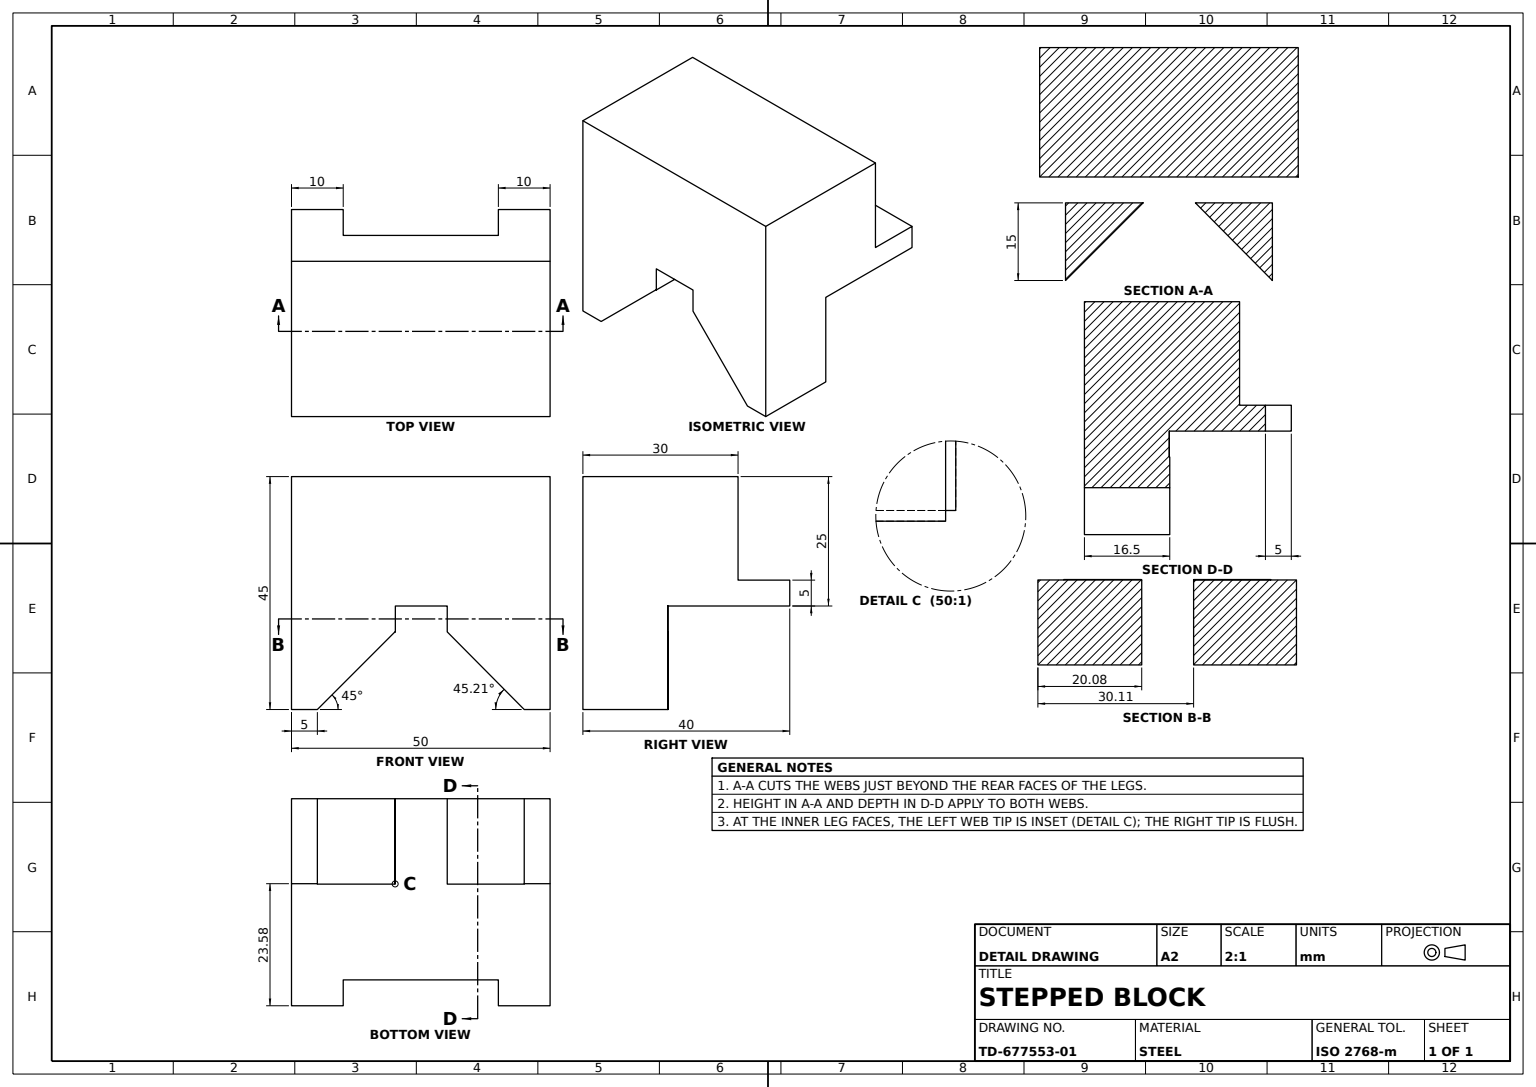
from build123d import *

# Parameters (mm, degrees)
BASE_BLOCK_SKETCH_W       = 50
BASE_BLOCK_SKETCH_H       = 30
BASE_BLOCK_50X30X25_DEPTH = 25
CORNER_STEP_5MM_DEPTH     = 5
LOWER_PLATE_SKETCH_W      = 19.888158271
LOWER_PLATE_SKETCH_H      = 16.417205811
LOWER_PLATE_5MM_DEPTH     = 5
LEG_SKETCH_W              = 5
LEG_SKETCH_H              = 16.417205811
LEG_15MM_DEPTH            = 15
TAPERED_WEB_16_5MM_DEPTH  = 16.5


with BuildPart() as part:
    # Base Block Sketch → Base Block 50x30x25 (new body)
    with BuildSketch(Plane(origin=(0, 0, 0), x_dir=(1, 0, 0), z_dir=(0, 1, 0))):
        with Locations((25, 15)):
            Rectangle(BASE_BLOCK_SKETCH_W, BASE_BLOCK_SKETCH_H)
    extrude(amount=BASE_BLOCK_50X30X25_DEPTH)

    # Corner Step Sketch → Corner Step 5mm (add)
    with BuildSketch(Plane(origin=(0, 0, 0), x_dir=(1, 0, 0), z_dir=(0, 1, 0))):
        Polygon((0, 30), (0, 40), (10, 40), (10, 35), (40, 35), (40, 40), (50, 40), (50, 30), (50, 0), (0, 0), align=None)
    extrude(amount=CORNER_STEP_5MM_DEPTH)

    # Lower Plate Sketch → Lower Plate 5mm (add)
    with BuildSketch(Plane.XZ):
        Polygon((6.770734002, 0), (0, 0), (0, -16.417205811), (6.770734002, -16.417205811), (20.078313967, -16.417205811), (20.078313967, 0), align=None)
        with Locations((40.055920865, -8.208602906)):
            Rectangle(LOWER_PLATE_SKETCH_W, LOWER_PLATE_SKETCH_H)
    extrude(amount=LOWER_PLATE_5MM_DEPTH)

    # Leg Sketch → Leg 15mm (add)
    with BuildSketch(Plane(origin=(0, -5, 0), x_dir=(-1, 0, 0), z_dir=(0, -1, 0))):
        with Locations((-2.5, 8.208602906)):
            Rectangle(LEG_SKETCH_W, LEG_SKETCH_H)
        with Locations((-47.5, 8.208602906)):
            Rectangle(LEG_SKETCH_W, LEG_SKETCH_H)
    extrude(amount=LEG_15MM_DEPTH)

    # Tapered Web Sketch → Tapered Web 16.5mm (add)
    with BuildSketch(Plane.XY):
        Polygon((30.111841729, -5), (45, -20), (45, -5), align=None)
        Polygon((5, -5), (5, -20), (20, -5), align=None)
    extrude(amount=-TAPERED_WEB_16_5MM_DEPTH)


solid = part.part
